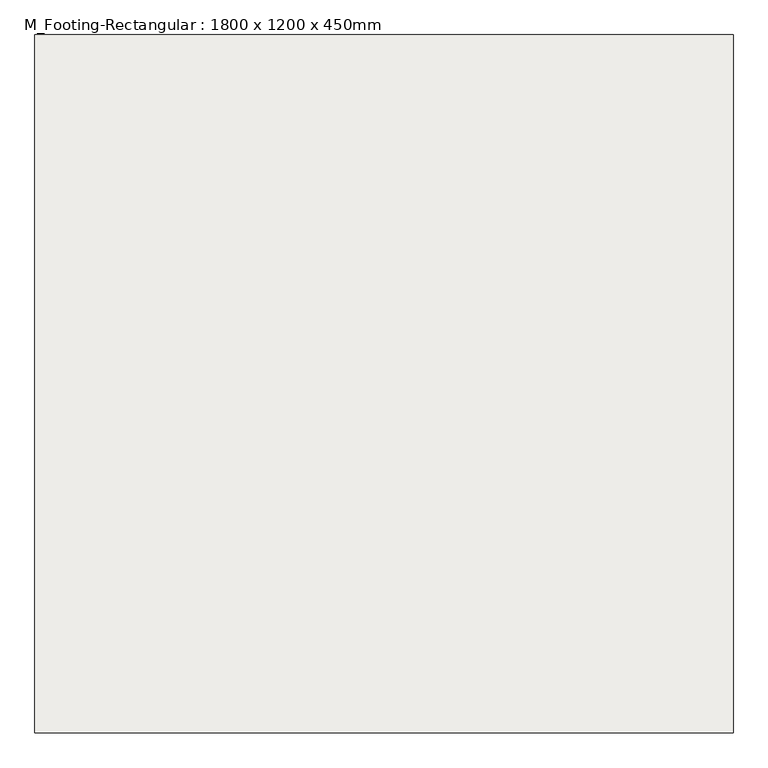
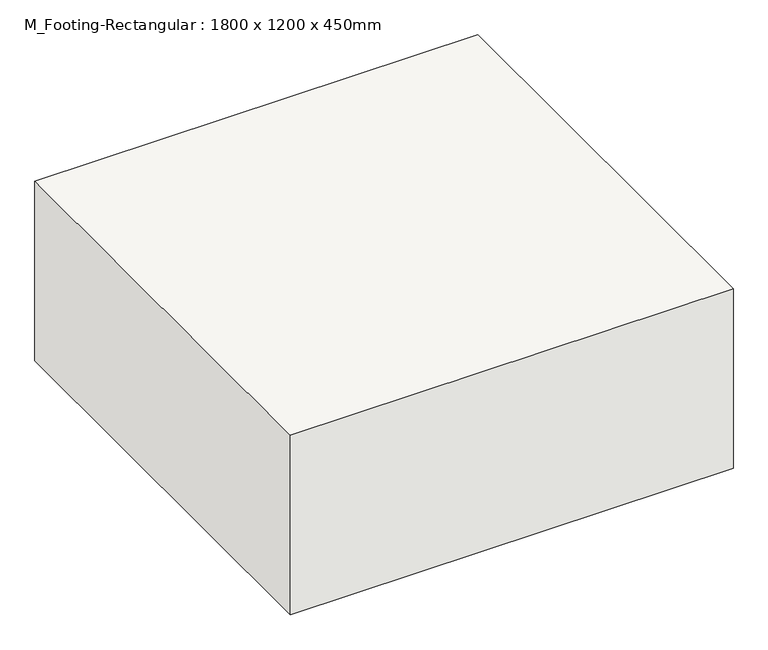
"""IFC4 building model written with IfcOpenShell, lengths in millimetres: slab geometry, M_Footing-Rectangular : 1800 x 1200 x 450mm."""

from ifc_helpers import new_model, si_unit, frame, origin, place, context, project, spatial, polyline, outline, extrude, source, transform, mapped, element, save


def m_footing_rectangular_1800_x_1200_x_450mm_ec84a8aa(model_context):
    return source(origin(), model_context, "Body", "SweptSolid", [
        extrude(outline(polyline([(1066.8, 1066.8), (1066.8, -1066.8), (-1066.8, -1066.8), (-1066.8, 1066.8), (1066.8, 1066.8)])), frame((0.0, 0.0, -914.4), z_axis=(0.0, 0.0, 1.0), x_axis=(1.0, 0.0, 0.0)), (0.0, 0.0, 1.0), 914.4),
    ])


if __name__ == "__main__":
    model = new_model("IFC4")
    model_context = context("Model", 3, world=origin())
    ifc_project = project(units=[si_unit("LENGTHUNIT", "METRE", prefix="MILLI")], contexts=[model_context])
    site = spatial("IfcSite", under=ifc_project)
    building = spatial("IfcBuilding", under=site)
    placement = place(None, origin())
    m_footing_rectangular_1800_x_1200_x_450mm_shape = m_footing_rectangular_1800_x_1200_x_450mm_ec84a8aa(model_context)
    element("IfcSlab", 1, ObjectType="M_Footing-Rectangular : 1800 x 1200 x 450mm", at=placement, inside=building, context=model_context, shape_type="MappedRepresentation", body=[
        mapped(m_footing_rectangular_1800_x_1200_x_450mm_shape, transform((0.0, 0.0, 0.0), x_axis=(1.0, 0.0, 0.0), y_axis=(0.0, 1.0, 0.0), z_axis=(0.0, 0.0, 1.0))),
    ])
    save(model, "model.ifc")

# Revit data of these elements
# Type "M_Footing-Rectangular : 1800 x 1200 x 450mm"
#   Width = 7' - 0"
#   Length = 7' - 0"
#   Foundation Thickness = 3' - 0"
#   Structural Material [instance default] = Concrete, Cast-in-Place gray
#   Assembly Code = ""
# Element 1 (IfcSlab, "M_Footing-Rectangular : 1800 x 1200 x 450mm")
#   Materials on its faces: "Concrete, Cast-in-Place gray"
# Materials
#   "Concrete, Cast-in-Place gray": class "Concrete", colour RGB 192 192 192, transparency 0, Description = "Cast-in-place concrete", Cost = 0
